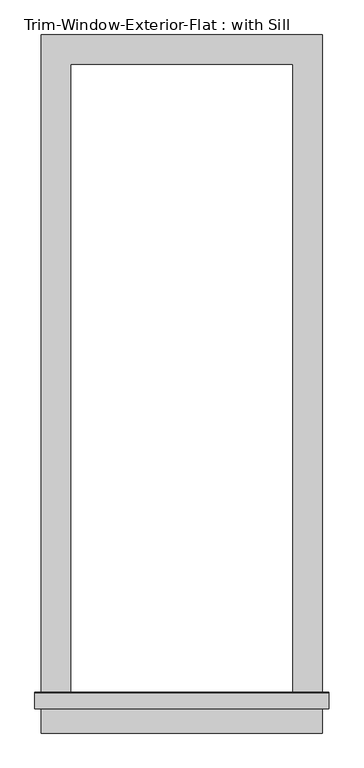
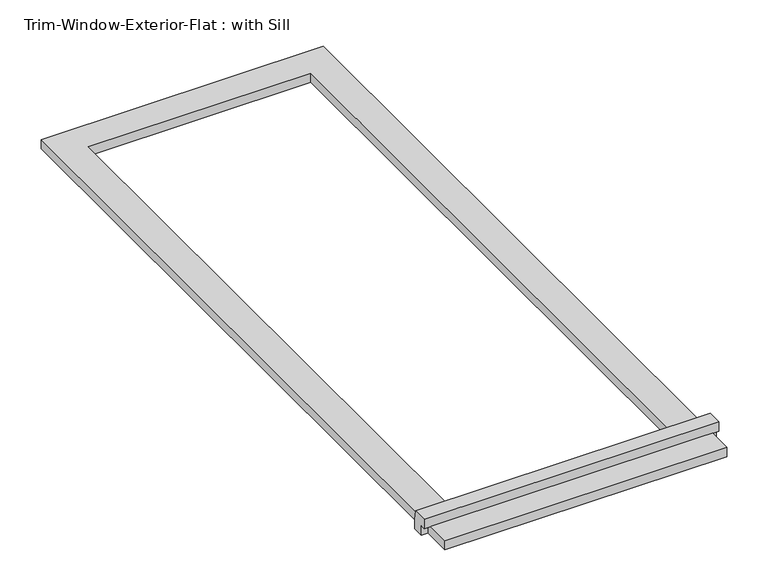
"""IFC4 building model written with IfcOpenShell, lengths in millimetres: proxy geometry, Trim-Window-Exterior-Flat : with Sill."""

from ifc_helpers import new_model, si_unit, frame, origin, origin_with_axes, place, context, project, spatial, polyline, outline, extrude, source, transform, mapped, element, save


def trim_window_exterior_flat_with_sill_499ee38d(model_context):
    return source(origin(), model_context, "Body", "SweptSolid", [
        extrude(outline(polyline([(273.05, -1241.3823709), (273.05, -1298.5323709), (-273.05, -1298.5323709), (-273.05, -1241.3823709), (273.05, -1241.3823709)])), origin_with_axes(), (0.0, 0.0, 1.0), 19.05),
        extrude(outline(polyline([(-1250.95, 38.1), (-1221.6580645, 38.1), (-1219.2, 19.05), (-1219.2, 0.0), (-1241.3823709, 0.0), (-1241.3823709, 19.05), (-1250.95, 19.05), (-1250.95, 38.1)])), frame((-285.75, 0.0, 0.0), z_axis=(1.0, 0.0, 0.0), x_axis=(0.0, 1.0, 0.0)), (0.0, 0.0, 1.0), 571.5),
        extrude(outline(polyline([(-273.05, 57.15), (273.05, 57.15), (273.05, -1219.2), (215.9, -1219.2), (215.9, 0.0), (-215.9, 0.0), (-215.9, -1219.2), (-273.05, -1219.2), (-273.05, 57.15)])), origin_with_axes(), (0.0, 0.0, 1.0), 19.05),
    ])


if __name__ == "__main__":
    model = new_model("IFC4")
    model_context = context("Model", 3, world=origin())
    ifc_project = project(units=[si_unit("LENGTHUNIT", "METRE", prefix="MILLI")], contexts=[model_context])
    site = spatial("IfcSite", under=ifc_project)
    building = spatial("IfcBuilding", under=site)
    placement = place(None, origin())
    trim_window_exterior_flat_with_sill_shape = trim_window_exterior_flat_with_sill_499ee38d(model_context)
    element("IfcBuildingElementProxy", 1, Name="Trim-Window-Exterior-Flat : with Sill", ObjectType="Trim-Window-Exterior-Flat : with Sill", at=placement, inside=building, context=model_context, shape_type="MappedRepresentation", body=[
        mapped(trim_window_exterior_flat_with_sill_shape, transform((0.0, 0.0, 0.0), x_axis=(1.0, 0.0, 0.0), y_axis=(0.0, 1.0, 0.0), z_axis=(0.0, 0.0, 1.0))),
    ])
    save(model, "model.ifc")

# Revit data of these elements
# Type "Trim-Window-Exterior-Flat : with Sill"
#   Trim Width = 0' - 2 1/4"
#   Trim Thickness_Picture Frame = 0' - 1 1/4"
#   Trim Thickness_with Sill = 0' - 0 3/4"
#   Sill Thickness = 0' - 1 1/4"
#   Opening Width [instance default] = 2' - 0"
#   Opening Height [instance default] = 3' - 0"
#   Default Elevation = 4' - 0"
#   Sill = yes
#   Picture Frame = no
#   Trim Material [instance default] = none
# Element 1 (IfcBuildingElementProxy, "Trim-Window-Exterior-Flat : with Sill")
#   Opening Width = 1' - 5"
#   Opening Height = 4' - 0"
#   Trim Material = Clad - White
#   Materials on its faces: "Clad - White"
# Materials
#   "Clad - White": class "Wood", colour RGB 242 242 238, transparency 0, Cost = 0
